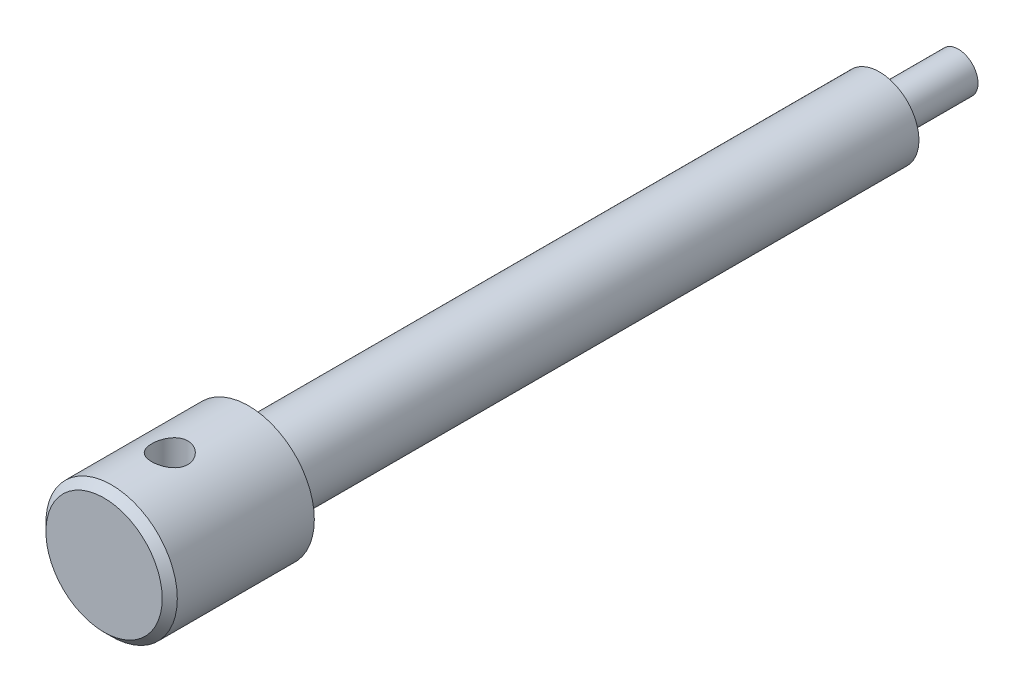
from build123d import *

# Parameters (mm, degrees)
HEAD_PROFILE_20_R          = 10
HEAD_20X22_DEPTH           = 22
SHANK_PROFILE_12_R         = 6
THREADED_SHANK_12X96_DEPTH = 96
PILOT_PROFILE_6_R          = 3
PILOT_TIP_6X12_DEPTH       = 12
CROSS_HOLE_PROFILE_5_5_R   = 2.75
CROSS_HOLE_5_5_DEPTH       = 12
HEAD_CHAMFER_1_15X45_SIZE  = 1.15


with BuildPart() as part:
    # Head Profile Ø20 → Head Ø20x22 (new body)
    with BuildSketch(Plane.XY):
        Circle(HEAD_PROFILE_20_R)
    extrude(amount=HEAD_20X22_DEPTH)

    # Shank Profile Ø12 → Threaded Shank Ø12x96 (add)
    with BuildSketch(Plane(origin=(0, 0, 0), x_dir=(-1, 0, 0), z_dir=(0, 0, -1))):
        Circle(SHANK_PROFILE_12_R)
    extrude(amount=THREADED_SHANK_12X96_DEPTH)

    # Pilot Profile Ø6 → Pilot Tip Ø6x12 (add)
    with BuildSketch(Plane(origin=(0, 0, -96), x_dir=(-1, 0, 0), z_dir=(0, 0, -1))):
        Circle(PILOT_PROFILE_6_R)
    extrude(amount=PILOT_TIP_6X12_DEPTH)

    # Cross Hole Profile Ø5.5 → Cross Hole Ø5.5 (cut, symmetric)
    with BuildSketch(Plane(origin=(0, 0, 0), x_dir=(1, 0, 0), z_dir=(0, 1, 0))):
        with Locations(Location((0, -12, 0), (0, 0, 270))):
            Circle(CROSS_HOLE_PROFILE_5_5_R)
    extrude(amount=CROSS_HOLE_5_5_DEPTH, both=True, mode=Mode.SUBTRACT)

    # Head Chamfer 1.15x45
    head_chamfer_1_15x45_edges = [part.edges().sort_by_distance(p)[0] for p in [
        (-10, 0, 22),
    ]]
    chamfer(head_chamfer_1_15x45_edges, length=HEAD_CHAMFER_1_15X45_SIZE)


solid = part.part
